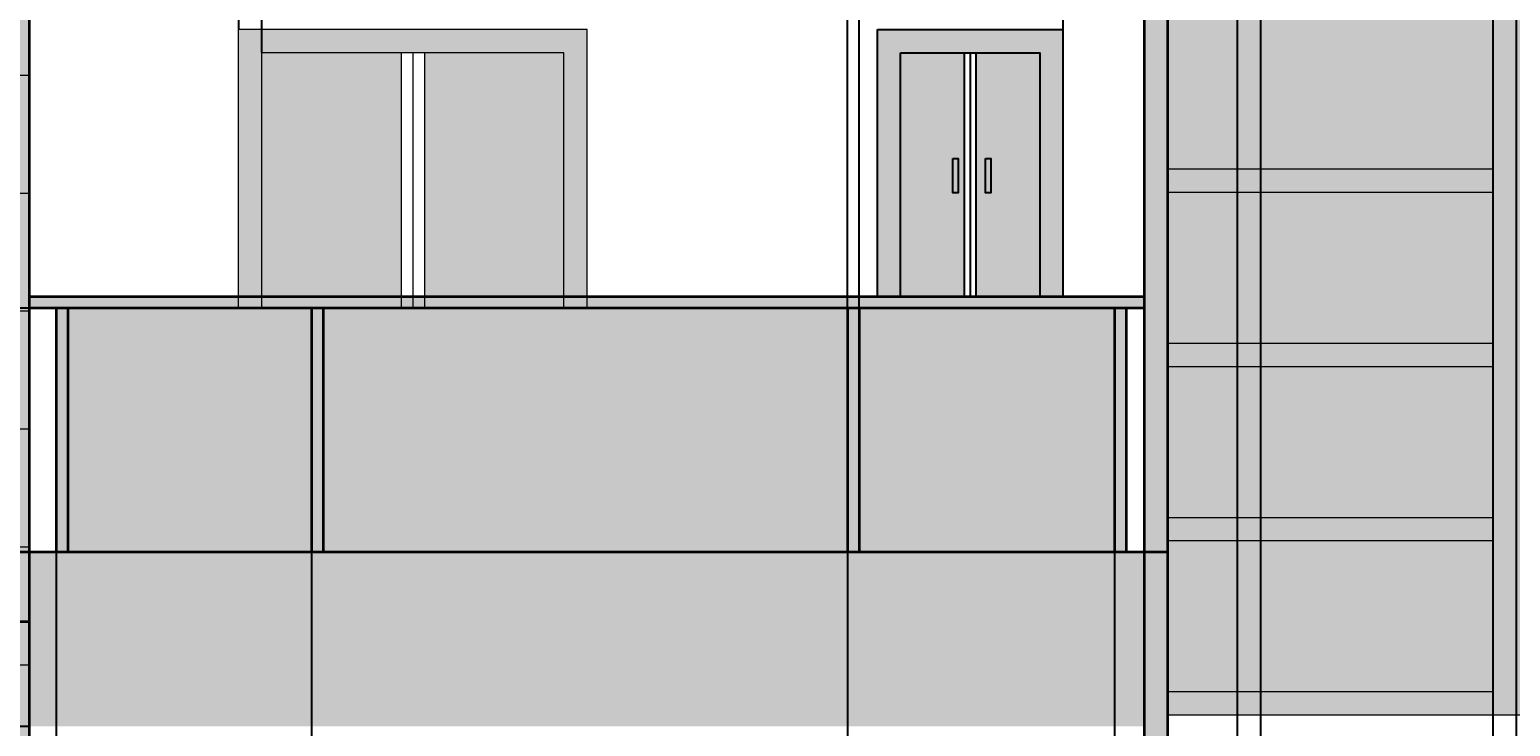
# Model space of a CAD drawing. Units: inches. Extents: x 2794 to 3619, y 522 to 1397.
# Tile 3 of 10: x 2954 to 3209, y 701 to 821. Entities that reach past the tile are written whole.
import ezdxf

# ---------------------------------------------------------------- set-up
doc = ezdxf.new("R2010")
doc.units = ezdxf.units.IN
for name, color, linetype, lineweight in [('A-ANNO-DIMS', 2, 'Continuous', 18), ('A-DOOR', 3, 'Continuous', 25), ('A-ELEV', 7, 'Continuous', 35), ('A-ELEV-PATT', 8, 'Continuous', 13), ('A-GLAZ', 4, 'Continuous', 18)]:
    doc.layers.add(name, color=color, linetype=linetype, lineweight=lineweight)
doc.styles.get("Standard").update_dxf_attribs({"font": 'arial.ttf'})
doc.dimstyles.get("Standard").update_dxf_attribs({"dimtxt": 0.18, "dimasz": 0.18, "dimexe": 0.18, "dimexo": 0.0625, "dimgap": 0.09, "dimtad": 0, "dimtih": 1, "dimtoh": 1, "dimdec": 4, "dimzin": 0, "dimdsep": 46, "dimtxsty": 'Standard', "dimcen": 0.09, "dimadec": 0, "dimazin": 0, "dimtfac": 1, "dimtdec": 4, "dimtofl": 0, "dimtmove": 0, "dimatfit": 3, "dimfxl": 1, "dimtolj": 1, "dimtzin": 0, "dimarcsym": 0})

# ---------------------------------------------------------------- blocks, each defined once
blk = doc.blocks.new('WIN-1500')
at = {"transparency": 33554646}
h = blk.add_hatch(color=256, dxfattribs=at)
h.dxf.hatch_style = 1
h.paths.add_polyline_path([(60, 48), (0, 48), (0, 2), (4, 2), (4, 44), (56, 44), (56, 2), (60, 2)])
at = {"transparency": 33554687}
h = blk.add_hatch(color=256, dxfattribs=at)
h.dxf.hatch_style = 1
h.set_gradient(color1=(248, 246, 176), color2=(74, 13, 14), name='INVCYLINDER')
h.paths.add_polyline_path([(56, 44), (32, 44), (32, 2), (56, 2)])
h.paths.add_polyline_path([(28, 44), (4, 44), (4, 2), (28, 2)])
for p, q in [((0, 0), (0, 48)), ((60, 48), (0, 48)), ((60, 0), (60, 48)), ((56, 44), (4, 44)), ((4, 0), (4, 44)), ((28, 44), (28, 0)), ((30, 44), (30, 0)), ((32, 44), (32, 0)), ((56, 0), (56, 44))]:
    blk.add_line(p, q)
blk = doc.blocks.new('DOOR-BALCONY-DBL')
at = {"transparency": 33554628}
h = blk.add_hatch(color=256, dxfattribs=at)
h.dxf.hatch_style = 1
h.paths.add_polyline_path([(4, 42), (28, 42), (28, 0), (32, 0), (32, 46), (0, 46), (0, 0), (4, 0)])
at = {"transparency": 33554646}
h = blk.add_hatch(color=256, dxfattribs=at)
h.dxf.hatch_style = 1
h.set_gradient(color1=(255, 255, 255), color2=(147, 149, 152), name='INVCYLINDER')
h.paths.add_polyline_path([(15, 42), (4, 42), (4, 0), (15, 0)])
h = blk.add_hatch(color=256, dxfattribs=at)
h.dxf.hatch_style = 1
h.set_gradient(color1=(255, 255, 255), color2=(147, 149, 152), name='INVCYLINDER')
h.paths.add_polyline_path([(28, 42), (17, 42), (17, 0), (28, 0)])
for p, q in [((0, 0), (0, 46)), ((0, 46), (32, 46)), ((4, 46), (28, 46)), ((32, 0), (32, 46)), ((4, 0), (4, 42)), ((4, 42), (28, 42)), ((15, 0), (15, 42)), ((16, 0), (16, 42)), ((17, 0), (17, 42)), ((28, 0), (28, 42))]:
    blk.add_line(p, q)
for points in [[(12.99, 23.83), (13.93, 23.83), (13.93, 17.87), (12.99, 17.87)], [(18.59, 23.83), (19.53, 23.83), (19.53, 17.87), (18.59, 17.87)]]:
    blk.add_lwpolyline(points, close=True)
blk = doc.blocks.new('*D16')
at = {"layer": 'A-ANNO-DIMS', "color": 0, "lineweight": -2, "transparency": 16777216}
for p, q in [((3142.2, 1356.64), (2793.99, 1356.64)), ((2794.17, 1356.46), (2794.17, 959.82)), ((2794.17, 562.82), (2794.17, 959.45)), ((2834.2, 562.64), (2793.99, 562.64))]:
    blk.add_line(p, q, dxfattribs=at)
at = {"layer": 'A-ANNO-DIMS', "color": 0, "transparency": 16777216}
for points in [[(2794.14, 1356.46), (2794.2, 1356.46), (2794.17, 1356.64)], [(2794.14, 562.82), (2794.2, 562.82), (2794.17, 562.64)]]:
    blk.add_solid(points, dxfattribs=at)
at = {"layer": 'Defpoints', "color": 0, "transparency": 16777216}
for p in [(2794.17, 1356.64), (3142.27, 1356.64), (2834.27, 562.64)]:
    blk.add_point(p, dxfattribs=at)
at = {"layer": 'A-ANNO-DIMS', "color": 0, "transparency": 16777216, "insert": (2794.17, 959.64), "char_height": 0.18, "attachment_point": 5}
blk.add_mtext('\\A1;794', dxfattribs=at)
blk = doc.blocks.new('*D29')
at = {"layer": 'A-ANNO-DIMS', "color": 0, "lineweight": -2, "transparency": 16777216}
for p, q in [((2990.27, 820.7), (2990.27, 1396.92)), ((2990.45, 1396.74), (2992.11, 1396.74)), ((2994.09, 1396.74), (2992.42, 1396.74)), ((2994.27, 816.7), (2994.27, 1396.92))]:
    blk.add_line(p, q, dxfattribs=at)
at = {"layer": 'A-ANNO-DIMS', "color": 0, "transparency": 16777216}
for points in [[(2990.45, 1396.77), (2990.45, 1396.71), (2990.27, 1396.74)], [(2994.09, 1396.77), (2994.09, 1396.71), (2994.27, 1396.74)]]:
    blk.add_solid(points, dxfattribs=at)
at = {"layer": 'Defpoints', "color": 0, "transparency": 16777216}
for p in [(2994.27, 1396.74), (2990.27, 820.64), (2994.27, 816.64)]:
    blk.add_point(p, dxfattribs=at)
at = {"layer": 'A-ANNO-DIMS', "color": 0, "transparency": 16777216, "insert": (2992.27, 1396.74), "char_height": 0.18, "attachment_point": 5}
blk.add_mtext('\\A1;4', dxfattribs=at)
blk = doc.blocks.new('*D31')
at = {"layer": 'A-ANNO-DIMS', "color": 0, "lineweight": -2, "transparency": 16777216}
for p, q in [((3132.27, 820.7), (3132.27, 1396.92)), ((3132.45, 1396.74), (3139.06, 1396.74)), ((3146.09, 1396.74), (3139.48, 1396.74)), ((3146.27, 774.7), (3146.27, 1396.92))]:
    blk.add_line(p, q, dxfattribs=at)
at = {"layer": 'A-ANNO-DIMS', "color": 0, "transparency": 16777216}
for points in [[(3132.45, 1396.77), (3132.45, 1396.71), (3132.27, 1396.74)], [(3146.09, 1396.77), (3146.09, 1396.71), (3146.27, 1396.74)]]:
    blk.add_solid(points, dxfattribs=at)
at = {"layer": 'Defpoints', "color": 0, "transparency": 16777216}
for p in [(3146.27, 1396.74), (3132.27, 820.64), (3146.27, 774.64)]:
    blk.add_point(p, dxfattribs=at)
at = {"layer": 'A-ANNO-DIMS', "color": 0, "transparency": 16777216, "insert": (3139.27, 1396.74), "char_height": 0.18, "attachment_point": 5}
blk.add_mtext('\\A1;14', dxfattribs=at)
blk = doc.blocks.new('*D32')
at = {"layer": 'A-ANNO-DIMS', "color": 0, "lineweight": -2, "transparency": 16777216}
for p, q in [((2954.27, 772.57), (2954.27, 522.36)), ((2958.83, 730.57), (2958.83, 522.36)), ((2954.45, 522.54), (2956.17, 522.54)), ((2958.65, 522.54), (2956.93, 522.54))]:
    blk.add_line(p, q, dxfattribs=at)
at = {"layer": 'A-ANNO-DIMS', "color": 0, "transparency": 16777216}
for points in [[(2954.45, 522.57), (2954.45, 522.51), (2954.27, 522.54)], [(2958.65, 522.57), (2958.65, 522.51), (2958.83, 522.54)]]:
    blk.add_solid(points, dxfattribs=at)
at = {"layer": 'Defpoints', "color": 0, "transparency": 16777216}
for p in [(2954.27, 772.64), (2958.83, 730.64), (2958.83, 522.54)]:
    blk.add_point(p, dxfattribs=at)
at = {"layer": 'A-ANNO-DIMS', "color": 0, "transparency": 16777216, "insert": (2956.55, 522.54), "char_height": 0.18, "attachment_point": 5}
blk.add_mtext('\\A1;4.561', dxfattribs=at)
blk = doc.blocks.new('*D33')
at = {"layer": 'A-ANNO-DIMS', "color": 0, "lineweight": -2, "transparency": 16777216}
for p, q in [((2958.83, 730.57), (2958.83, 522.36)), ((3002.83, 730.57), (3002.83, 522.36)), ((2959.01, 522.54), (2980.6, 522.54)), ((3002.65, 522.54), (2981.05, 522.54))]:
    blk.add_line(p, q, dxfattribs=at)
at = {"layer": 'A-ANNO-DIMS', "color": 0, "transparency": 16777216}
for points in [[(2959.01, 522.57), (2959.01, 522.51), (2958.83, 522.54)], [(3002.65, 522.57), (3002.65, 522.51), (3002.83, 522.54)]]:
    blk.add_solid(points, dxfattribs=at)
at = {"layer": 'Defpoints', "color": 0, "transparency": 16777216}
for p in [(2958.83, 730.64), (3002.83, 730.64), (3002.83, 522.54)]:
    blk.add_point(p, dxfattribs=at)
at = {"layer": 'A-ANNO-DIMS', "color": 0, "transparency": 16777216, "insert": (2980.83, 522.54), "char_height": 0.18, "attachment_point": 5}
blk.add_mtext('\\A1;44', dxfattribs=at)
blk = doc.blocks.new('*D34')
at = {"layer": 'A-ANNO-DIMS', "color": 0, "lineweight": -2, "transparency": 16777216}
for p, q in [((3002.83, 730.57), (3002.83, 522.36)), ((3095.13, 730.57), (3095.13, 522.36)), ((3003.01, 522.54), (3048.66, 522.54)), ((3094.95, 522.54), (3049.3, 522.54))]:
    blk.add_line(p, q, dxfattribs=at)
at = {"layer": 'A-ANNO-DIMS', "color": 0, "transparency": 16777216}
for points in [[(3003.01, 522.57), (3003.01, 522.51), (3002.83, 522.54)], [(3094.95, 522.57), (3094.95, 522.51), (3095.13, 522.54)]]:
    blk.add_solid(points, dxfattribs=at)
at = {"layer": 'Defpoints', "color": 0, "transparency": 16777216}
for p in [(3002.83, 730.64), (3095.13, 730.64), (3095.13, 522.54)]:
    blk.add_point(p, dxfattribs=at)
at = {"layer": 'A-ANNO-DIMS', "color": 0, "transparency": 16777216, "insert": (3048.98, 522.54), "char_height": 0.18, "attachment_point": 5}
blk.add_mtext('\\A1;92.3', dxfattribs=at)
blk = doc.blocks.new('*D35')
at = {"layer": 'A-ANNO-DIMS', "color": 0, "lineweight": -2, "transparency": 16777216}
for p, q in [((3095.13, 730.57), (3095.13, 522.36)), ((3141.11, 730.57), (3141.11, 522.36)), ((3095.31, 522.54), (3117.72, 522.54)), ((3140.93, 522.54), (3118.52, 522.54))]:
    blk.add_line(p, q, dxfattribs=at)
at = {"layer": 'A-ANNO-DIMS', "color": 0, "transparency": 16777216}
for points in [[(3095.31, 522.57), (3095.31, 522.51), (3095.13, 522.54)], [(3140.93, 522.57), (3140.93, 522.51), (3141.11, 522.54)]]:
    blk.add_solid(points, dxfattribs=at)
at = {"layer": 'Defpoints', "color": 0, "transparency": 16777216}
for p in [(3095.13, 730.64), (3141.11, 730.64), (3141.11, 522.54)]:
    blk.add_point(p, dxfattribs=at)
at = {"layer": 'A-ANNO-DIMS', "color": 0, "transparency": 16777216, "insert": (3118.12, 522.54), "char_height": 0.18, "attachment_point": 5}
blk.add_mtext('\\A1;45.98', dxfattribs=at)
blk = doc.blocks.new('*D36')
at = {"layer": 'A-ANNO-DIMS', "color": 0, "lineweight": -2, "transparency": 16777216}
for p, q in [((3146.27, 772.57), (3146.27, 522.36)), ((3141.11, 730.57), (3141.11, 522.36)), ((3141.29, 522.54), (3143.3, 522.54)), ((3146.09, 522.54), (3144.08, 522.54))]:
    blk.add_line(p, q, dxfattribs=at)
at = {"layer": 'A-ANNO-DIMS', "color": 0, "transparency": 16777216}
for points in [[(3141.29, 522.57), (3141.29, 522.51), (3141.11, 522.54)], [(3146.09, 522.57), (3146.09, 522.51), (3146.27, 522.54)]]:
    blk.add_solid(points, dxfattribs=at)
at = {"layer": 'Defpoints', "color": 0, "transparency": 16777216}
for p in [(3146.27, 772.64), (3141.11, 730.64), (3146.27, 522.54)]:
    blk.add_point(p, dxfattribs=at)
at = {"layer": 'A-ANNO-DIMS', "color": 0, "transparency": 16777216, "insert": (3143.69, 522.54), "char_height": 0.18, "attachment_point": 5}
blk.add_mtext('\\A1;5.154', dxfattribs=at)
blk = doc.blocks.new('*D37')
at = {"layer": 'A-ANNO-DIMS', "color": 0, "lineweight": -2, "transparency": 16777216}
for p, q in [((3095.13, 772.7), (3095.13, 1396.92)), ((3095.31, 1396.74), (3095.98, 1396.74)), ((3096.95, 1396.74), (3096.28, 1396.74)), ((3097.13, 772.7), (3097.13, 1396.92))]:
    blk.add_line(p, q, dxfattribs=at)
at = {"layer": 'A-ANNO-DIMS', "color": 0, "transparency": 16777216}
for points in [[(3095.31, 1396.77), (3095.31, 1396.71), (3095.13, 1396.74)], [(3096.95, 1396.77), (3096.95, 1396.71), (3097.13, 1396.74)]]:
    blk.add_solid(points, dxfattribs=at)
at = {"layer": 'Defpoints', "color": 0, "transparency": 16777216}
for p in [(3097.13, 1396.74), (3095.13, 772.64), (3097.13, 772.64)]:
    blk.add_point(p, dxfattribs=at)
at = {"layer": 'A-ANNO-DIMS', "color": 0, "transparency": 16777216, "insert": (3096.13, 1396.74), "char_height": 0.18, "attachment_point": 5}
blk.add_mtext('\\A1;2', dxfattribs=at)
blk = doc.blocks.new('*D38')
at = {"layer": 'A-ANNO-DIMS', "color": 0, "lineweight": -2, "transparency": 16777216}
for p, q in [((2958.76, 730.64), (2793.99, 730.64)), ((2794.17, 730.46), (2794.17, 715.82)), ((2794.17, 700.82), (2794.17, 715.45)), ((2954.2, 700.64), (2793.99, 700.64))]:
    blk.add_line(p, q, dxfattribs=at)
at = {"layer": 'A-ANNO-DIMS', "color": 0, "transparency": 16777216}
for points in [[(2794.14, 730.46), (2794.2, 730.46), (2794.17, 730.64)], [(2794.14, 700.82), (2794.2, 700.82), (2794.17, 700.64)]]:
    blk.add_solid(points, dxfattribs=at)
at = {"layer": 'Defpoints', "color": 0, "transparency": 16777216}
for p in [(2794.17, 730.64), (2958.83, 730.64), (2954.27, 700.64)]:
    blk.add_point(p, dxfattribs=at)
at = {"layer": 'A-ANNO-DIMS', "color": 0, "transparency": 16777216, "insert": (2794.17, 715.64), "char_height": 0.18, "attachment_point": 5}
blk.add_mtext('\\A1;30', dxfattribs=at)
blk = doc.blocks.new('*D39')
at = {"layer": 'A-ANNO-DIMS', "color": 0, "lineweight": -2, "transparency": 16777216}
for p, q in [((2954.2, 772.64), (2793.99, 772.64)), ((2794.17, 772.46), (2794.17, 751.82)), ((2794.17, 730.82), (2794.17, 751.45)), ((2958.76, 730.64), (2793.99, 730.64))]:
    blk.add_line(p, q, dxfattribs=at)
at = {"layer": 'A-ANNO-DIMS', "color": 0, "transparency": 16777216}
for points in [[(2794.14, 772.46), (2794.2, 772.46), (2794.17, 772.64)], [(2794.14, 730.82), (2794.2, 730.82), (2794.17, 730.64)]]:
    blk.add_solid(points, dxfattribs=at)
at = {"layer": 'Defpoints', "color": 0, "transparency": 16777216}
for p in [(2794.17, 772.64), (2954.27, 772.64), (2958.83, 730.64)]:
    blk.add_point(p, dxfattribs=at)
at = {"layer": 'A-ANNO-DIMS', "color": 0, "transparency": 16777216, "insert": (2794.17, 751.64), "char_height": 0.18, "attachment_point": 5}
blk.add_mtext('\\A1;42', dxfattribs=at)
blk = doc.blocks.new('*D49')
at = {"layer": 'A-ANNO-DIMS', "color": 0, "lineweight": -2, "transparency": 16777216}
for p, q in [((3146.27, 1256.19), (3146.27, 522.36)), ((3150.27, 1254.57), (3150.27, 522.36)), ((3146.45, 522.54), (3148.11, 522.54)), ((3150.09, 522.54), (3148.42, 522.54))]:
    blk.add_line(p, q, dxfattribs=at)
at = {"layer": 'A-ANNO-DIMS', "color": 0, "transparency": 16777216}
for points in [[(3146.45, 522.57), (3146.45, 522.51), (3146.27, 522.54)], [(3150.09, 522.57), (3150.09, 522.51), (3150.27, 522.54)]]:
    blk.add_solid(points, dxfattribs=at)
at = {"layer": 'Defpoints', "color": 0, "transparency": 16777216}
for p in [(3146.27, 1256.25), (3150.27, 1254.64), (3150.27, 522.54)]:
    blk.add_point(p, dxfattribs=at)
at = {"layer": 'A-ANNO-DIMS', "color": 0, "transparency": 16777216, "insert": (3148.27, 522.54), "char_height": 0.18, "attachment_point": 5}
blk.add_mtext('\\A1;4', dxfattribs=at)
blk = doc.blocks.new('*D50')
at = {"layer": 'A-ANNO-DIMS', "color": 0, "lineweight": -2, "transparency": 16777216}
for p, q in [((3150.27, 1254.57), (3150.27, 522.36)), ((3206.27, 1254.57), (3206.27, 522.36)), ((3150.45, 522.54), (3178.05, 522.54)), ((3206.09, 522.54), (3178.48, 522.54))]:
    blk.add_line(p, q, dxfattribs=at)
at = {"layer": 'A-ANNO-DIMS', "color": 0, "transparency": 16777216}
for points in [[(3150.45, 522.57), (3150.45, 522.51), (3150.27, 522.54)], [(3206.09, 522.57), (3206.09, 522.51), (3206.27, 522.54)]]:
    blk.add_solid(points, dxfattribs=at)
at = {"layer": 'Defpoints', "color": 0, "transparency": 16777216}
for p in [(3150.27, 1254.64), (3206.27, 1254.64), (3206.27, 522.54)]:
    blk.add_point(p, dxfattribs=at)
at = {"layer": 'A-ANNO-DIMS', "color": 0, "transparency": 16777216, "insert": (3178.27, 522.54), "char_height": 0.18, "attachment_point": 5}
blk.add_mtext('\\A1;56', dxfattribs=at)
blk = doc.blocks.new('*D51')
at = {"layer": 'A-ANNO-DIMS', "color": 0, "lineweight": -2, "transparency": 16777216}
for p, q in [((3206.27, 1254.57), (3206.27, 522.36)), ((3210.27, 1254.57), (3210.27, 522.36)), ((3206.45, 522.54), (3208.11, 522.54)), ((3210.09, 522.54), (3208.42, 522.54))]:
    blk.add_line(p, q, dxfattribs=at)
at = {"layer": 'A-ANNO-DIMS', "color": 0, "transparency": 16777216}
for points in [[(3206.45, 522.57), (3206.45, 522.51), (3206.27, 522.54)], [(3210.09, 522.57), (3210.09, 522.51), (3210.27, 522.54)]]:
    blk.add_solid(points, dxfattribs=at)
at = {"layer": 'Defpoints', "color": 0, "transparency": 16777216}
for p in [(3206.27, 1254.64), (3210.27, 1254.64), (3210.27, 522.54)]:
    blk.add_point(p, dxfattribs=at)
at = {"layer": 'A-ANNO-DIMS', "color": 0, "transparency": 16777216, "insert": (3208.27, 522.54), "char_height": 0.18, "attachment_point": 5}
blk.add_mtext('\\A1;4', dxfattribs=at)
blk = doc.blocks.new('*D56')
at = {"layer": 'A-ANNO-DIMS', "color": 0, "lineweight": -2, "transparency": 16777216}
for p, q in [((3162.27, 664.7), (3162.27, 1396.92)), ((3162.45, 1396.74), (3206.05, 1396.74)), ((3250.09, 1396.74), (3206.49, 1396.74)), ((3250.27, 664.7), (3250.27, 1396.92))]:
    blk.add_line(p, q, dxfattribs=at)
at = {"layer": 'A-ANNO-DIMS', "color": 0, "transparency": 16777216}
for points in [[(3162.45, 1396.77), (3162.45, 1396.71), (3162.27, 1396.74)], [(3250.09, 1396.77), (3250.09, 1396.71), (3250.27, 1396.74)]]:
    blk.add_solid(points, dxfattribs=at)
at = {"layer": 'Defpoints', "color": 0, "transparency": 16777216}
for p in [(3250.27, 1396.74), (3162.27, 664.64), (3250.27, 664.64)]:
    blk.add_point(p, dxfattribs=at)
at = {"layer": 'A-ANNO-DIMS', "color": 0, "transparency": 16777216, "insert": (3206.27, 1396.74), "char_height": 0.18, "attachment_point": 5}
blk.add_mtext('\\A1;88', dxfattribs=at)
blk = doc.blocks.new('*D57')
at = {"layer": 'A-ANNO-DIMS', "color": 0, "lineweight": -2, "transparency": 16777216}
for p, q in [((3162.27, 664.7), (3162.27, 1396.92)), ((3162.45, 1396.74), (3164.11, 1396.74)), ((3166.09, 1396.74), (3164.42, 1396.74)), ((3166.27, 660.7), (3166.27, 1396.92))]:
    blk.add_line(p, q, dxfattribs=at)
at = {"layer": 'A-ANNO-DIMS', "color": 0, "transparency": 16777216}
for points in [[(3162.45, 1396.77), (3162.45, 1396.71), (3162.27, 1396.74)], [(3166.09, 1396.77), (3166.09, 1396.71), (3166.27, 1396.74)]]:
    blk.add_solid(points, dxfattribs=at)
at = {"layer": 'Defpoints', "color": 0, "transparency": 16777216}
for p in [(3166.27, 1396.74), (3162.27, 664.64), (3166.27, 660.64)]:
    blk.add_point(p, dxfattribs=at)
at = {"layer": 'A-ANNO-DIMS', "color": 0, "transparency": 16777216, "insert": (3164.27, 1396.74), "char_height": 0.18, "attachment_point": 5}
blk.add_mtext('\\A1;4', dxfattribs=at)
blk = doc.blocks.new('*D58')
at = {"layer": 'A-ANNO-DIMS', "color": 0, "lineweight": -2, "transparency": 16777216}
for p, q in [((3150.27, 580.7), (3150.27, 1396.92)), ((3150.45, 1396.74), (3156.06, 1396.74)), ((3162.09, 1396.74), (3156.48, 1396.74)), ((3162.27, 664.7), (3162.27, 1396.92))]:
    blk.add_line(p, q, dxfattribs=at)
at = {"layer": 'A-ANNO-DIMS', "color": 0, "transparency": 16777216}
for points in [[(3150.45, 1396.77), (3150.45, 1396.71), (3150.27, 1396.74)], [(3162.09, 1396.77), (3162.09, 1396.71), (3162.27, 1396.74)]]:
    blk.add_solid(points, dxfattribs=at)
at = {"layer": 'Defpoints', "color": 0, "transparency": 16777216}
for p in [(3162.27, 1396.74), (3162.27, 664.64), (3150.27, 580.64)]:
    blk.add_point(p, dxfattribs=at)
at = {"layer": 'A-ANNO-DIMS', "color": 0, "transparency": 16777216, "insert": (3156.27, 1396.74), "char_height": 0.18, "attachment_point": 5}
blk.add_mtext('\\A1;12', dxfattribs=at)

msp = doc.modelspace()

# ---------------------------------------------------------------- hatches: boundary and pattern name
at = {"layer": 'A-ELEV-PATT', "transparency": 33554687}
h = msp.add_hatch(color=256, dxfattribs=at)
h.dxf.hatch_style = 1
h.paths.add_polyline_path([(3262.2659, 1350.6351), (3150.2659, 1350.6351), (3150.2659, 1279.0155, -0.68639605), (3262.2659, 1279.0155)])
h.paths.add_polyline_path([(3210.2659, 1314.1121), (3210.2659, 1258.6351), (3262.2659, 1258.6351, 0.39146256)])
h.paths.add_polyline_path([(3206.2659, 1314.2551, 0.41222069), (3150.2659, 1258.6351), (3206.2659, 1258.6351)])
h.paths.add_polyline_path([(3262.2659, 1254.6351), (3210.2659, 1254.6351), (3210.2659, 1216.6351), (3262.2659, 1216.6351)])
h.paths.add_polyline_path([(3206.2659, 1254.6351), (3150.2659, 1254.6351), (3150.2659, 1216.6351), (3206.2659, 1216.6351)])
h.paths.add_polyline_path([(3262.2659, 1212.6351), (3210.2659, 1212.6351), (3210.2659, 1186.6351), (3262.2659, 1186.6351)])
h.paths.add_polyline_path([(3206.2659, 1212.6351), (3150.2659, 1212.6351), (3150.2659, 1186.6351), (3206.2659, 1186.6351)])
h.paths.add_polyline_path([(3206.2659, 1182.6351), (3150.2659, 1182.6351), (3150.2659, 1156.6351), (3206.2659, 1156.6351)])
h.paths.add_polyline_path([(3262.2659, 1182.6351), (3210.2659, 1182.6351), (3210.2659, 1156.6351), (3262.2659, 1156.6351)])
h.paths.add_polyline_path([(3262.2659, 1152.6351), (3210.2659, 1152.6351), (3210.2659, 1126.6351), (3262.2659, 1126.6351)])
h.paths.add_polyline_path([(3206.2659, 1152.6351), (3150.2659, 1152.6351), (3150.2659, 1126.6351), (3206.2659, 1126.6351)])
h.paths.add_polyline_path([(3262.2659, 1122.6351), (3210.2659, 1122.6351), (3210.2659, 1096.6351), (3262.2659, 1096.6351)])
h.paths.add_polyline_path([(3206.2659, 1122.6351), (3150.2659, 1122.6351), (3150.2659, 1096.6351), (3206.2659, 1096.6351)])
h.paths.add_polyline_path([(3206.2659, 1092.6351), (3150.2659, 1092.6351), (3150.2659, 1066.6351), (3206.2659, 1066.6351)])
h.paths.add_polyline_path([(3262.2659, 1092.6351), (3210.2659, 1092.6351), (3210.2659, 1066.6351), (3262.2659, 1066.6351)])
h.paths.add_polyline_path([(3262.2659, 1062.6351), (3210.2659, 1062.6351), (3210.2659, 1036.6351), (3262.2659, 1036.6351)])
h.paths.add_polyline_path([(3206.2659, 1062.6351), (3150.2659, 1062.6351), (3150.2659, 1036.6351), (3206.2659, 1036.6351)])
h.paths.add_polyline_path([(3206.2659, 1032.6351), (3150.2659, 1032.6351), (3150.2659, 1006.6351), (3206.2659, 1006.6351)])
h.paths.add_polyline_path([(3262.2659, 1032.6351), (3210.2659, 1032.6351), (3210.2659, 1006.6351), (3262.2659, 1006.6351)])
h.paths.add_polyline_path([(3262.2659, 1002.6351), (3210.2659, 1002.6351), (3210.2659, 976.6351), (3262.2659, 976.6351)])
h.paths.add_polyline_path([(3206.2659, 1002.6351), (3150.2659, 1002.6351), (3150.2659, 976.6351), (3206.2659, 976.6351)])
h.paths.add_polyline_path([(3206.2659, 972.6351), (3150.2659, 972.6351), (3150.2659, 946.6351), (3206.2659, 946.6351)])
h.paths.add_polyline_path([(3206.2659, 942.6351), (3150.2659, 942.6351), (3150.2659, 916.6351), (3206.2659, 916.6351)])
h.paths.add_polyline_path([(3262.2659, 942.6351), (3210.2659, 942.6351), (3210.2659, 916.6351), (3262.2659, 916.6351)])
h.paths.add_polyline_path([(3262.2659, 972.6351), (3210.2659, 972.6351), (3210.2659, 946.6351), (3262.2659, 946.6351)])
h.paths.add_polyline_path([(3262.2659, 912.6351), (3210.2659, 912.6351), (3210.2659, 886.6351), (3262.2659, 886.6351)])
h.paths.add_polyline_path([(3206.2659, 912.6351), (3150.2659, 912.6351), (3150.2659, 886.6351), (3206.2659, 886.6351)])
h.paths.add_polyline_path([(3206.2659, 882.6351), (3150.2659, 882.6351), (3150.2659, 856.6351), (3206.2659, 856.6351)])
h.paths.add_polyline_path([(3262.2659, 882.6351), (3210.2659, 882.6351), (3210.2659, 856.6351), (3262.2659, 856.6351)])
h.paths.add_polyline_path([(3262.2659, 852.6351), (3210.2659, 852.6351), (3210.2659, 826.6351), (3262.2659, 826.6351)])
h.paths.add_polyline_path([(3206.2659, 852.6351), (3150.2659, 852.6351), (3150.2659, 826.6351), (3206.2659, 826.6351)])
h.paths.add_polyline_path([(3206.2659, 822.6351), (3150.2659, 822.6351), (3150.2659, 796.6351), (3206.2659, 796.6351)])
h.paths.add_polyline_path([(3262.2659, 822.6351), (3210.2659, 822.6351), (3210.2659, 796.6351), (3262.2659, 796.6351)])
h.paths.add_polyline_path([(3262.2659, 792.6351), (3210.2659, 792.6351), (3210.2659, 766.6351), (3262.2659, 766.6351)])
h.paths.add_polyline_path([(3206.2659, 792.6351), (3150.2659, 792.6351), (3150.2659, 766.6351), (3206.2659, 766.6351)])
h.paths.add_polyline_path([(3206.2659, 762.6351), (3150.2659, 762.6351), (3150.2659, 736.6351), (3206.2659, 736.6351)])
h.paths.add_polyline_path([(3206.2659, 732.6351), (3150.2659, 732.6351), (3150.2659, 706.6351), (3206.2659, 706.6351)])
h.paths.add_polyline_path([(3262.2659, 732.6351), (3210.2659, 732.6351), (3210.2659, 706.6351), (3262.2659, 706.6351)])
h.paths.add_polyline_path([(3262.2659, 762.6351), (3210.2659, 762.6351), (3210.2659, 736.6351), (3262.2659, 736.6351)])
h = msp.add_hatch(color=256, dxfattribs=at)
h.dxf.hatch_style = 1
h.paths.add_polyline_path([(3150.2659, 1257.8725, -0.00340445), (3150.2659, 1258.6351), (3146.2659, 1258.6351), (3146.2659, 1228.6351), (3150.2659, 1228.6351)])
h.paths.add_polyline_path([(3262.2659, 1258.6351), (3210.2659, 1258.6351), (3210.2659, 1314.1121, 0.01787385), (3206.2659, 1314.2551), (3206.2659, 1258.6351), (3150.2659, 1258.6351), (3150.2659, 1254.6351), (3206.2659, 1254.6351), (3206.2659, 1216.6351), (3150.2659, 1216.6351), (3150.2659, 1212.6351), (3206.2659, 1212.6351), (3206.2659, 1186.6351), (3150.2659, 1186.6351), (3150.2659, 1182.6351), (3206.2659, 1182.6351), (3206.2659, 1156.6351), (3150.2659, 1156.6351), (3150.2659, 1152.6351), (3206.2659, 1152.6351), (3206.2659, 1126.6351), (3150.2659, 1126.6351), (3150.2659, 1122.6351), (3206.2659, 1122.6351), (3206.2659, 1096.6351), (3150.2659, 1096.6351), (3150.2659, 1092.6351), (3206.2659, 1092.6351), (3206.2659, 1066.6351), (3150.2659, 1066.6351), (3150.2659, 1062.6351), (3206.2659, 1062.6351), (3206.2659, 1036.6351), (3150.2659, 1036.6351), (3150.2659, 1032.6351), (3206.2659, 1032.6351), (3206.2659, 1006.6351), (3150.2659, 1006.6351), (3150.2659, 1002.6351), (3206.2659, 1002.6351), (3206.2659, 976.6351), (3150.2659, 976.6351), (3150.2659, 972.6351), (3206.2659, 972.6351), (3206.2659, 946.6351), (3150.2659, 946.6351), (3150.2659, 942.6351), (3206.2659, 942.6351), (3206.2659, 916.6351), (3150.2659, 916.6351), (3150.2659, 912.6351), (3206.2659, 912.6351), (3206.2659, 886.6351), (3150.2659, 886.6351), (3150.2659, 882.6351), (3206.2659, 882.6351), (3206.2659, 856.6351), (3150.2659, 856.6351), (3150.2659, 852.6351), (3206.2659, 852.6351), (3206.2659, 826.6351), (3150.2659, 826.6351), (3150.2659, 822.6351), (3206.2659, 822.6351), (3206.2659, 796.6351), (3150.2659, 796.6351), (3150.2659, 792.6351), (3206.2659, 792.6351), (3206.2659, 766.6351), (3150.2659, 766.6351), (3150.2659, 762.6351), (3206.2659, 762.6351), (3206.2659, 736.6351), (3150.2659, 736.6351), (3150.2659, 732.6351), (3206.2659, 732.6351), (3206.2659, 706.6351), (3150.2659, 706.6351), (3150.2659, 702.6351), (3262.2659, 702.6351), (3262.2659, 706.6351), (3210.2659, 706.6351), (3210.2659, 732.6351), (3262.2659, 732.6351), (3262.2659, 736.6351), (3210.2659, 736.6351), (3210.2659, 762.6351), (3262.2659, 762.6351), (3262.2659, 766.6351), (3210.2659, 766.6351), (3210.2659, 792.6351), (3262.2659, 792.6351), (3262.2659, 796.6351), (3210.2659, 796.6351), (3210.2659, 822.6351), (3262.2659, 822.6351), (3262.2659, 826.6351), (3210.2659, 826.6351), (3210.2659, 852.6351), (3262.2659, 852.6351), (3262.2659, 856.6351), (3210.2659, 856.6351), (3210.2659, 882.6351), (3262.2659, 882.6351), (3262.2659, 886.6351), (3210.2659, 886.6351), (3210.2659, 912.6351), (3262.2659, 912.6351), (3262.2659, 916.6351), (3210.2659, 916.6351), (3210.2659, 942.6351), (3262.2659, 942.6351), (3262.2659, 946.6351), (3210.2659, 946.6351), (3210.2659, 972.6351), (3262.2659, 972.6351), (3262.2659, 976.6351), (3210.2659, 976.6351), (3210.2659, 1002.6351), (3262.2659, 1002.6351), (3262.2659, 1006.6351), (3210.2659, 1006.6351), (3210.2659, 1032.6351), (3262.2659, 1032.6351), (3262.2659, 1036.6351), (3210.2659, 1036.6351), (3210.2659, 1062.6351), (3262.2659, 1062.6351), (3262.2659, 1066.6351), (3210.2659, 1066.6351), (3210.2659, 1092.6351), (3262.2659, 1092.6351), (3262.2659, 1096.6351), (3210.2659, 1096.6351), (3210.2659, 1122.6351), (3262.2659, 1122.6351), (3262.2659, 1126.6351), (3210.2659, 1126.6351), (3210.2659, 1152.6351), (3262.2659, 1152.6351), (3262.2659, 1156.6351), (3210.2659, 1156.6351), (3210.2659, 1182.6351), (3262.2659, 1182.6351), (3262.2659, 1186.6351), (3210.2659, 1186.6351), (3210.2659, 1212.6351), (3262.2659, 1212.6351), (3262.2659, 1216.6351), (3210.2659, 1216.6351), (3210.2659, 1254.6351), (3262.2659, 1254.6351)])
h = msp.add_hatch(color=256, dxfattribs=at)
h.dxf.hatch_style = 1
h.paths.add_polyline_path([(2852.2659, 1246.6351), (2954.2659, 1246.6351), (2954.2659, 1258.6351), (2900.2659, 1258.6351), (2900.2659, 1294.6351), (2852.2659, 1294.6351)])
h.paths.add_polyline_path([(3512.2659, 1294.6351), (3512.2659, 1258.6351), (3458.2659, 1258.6351), (3458.2659, 1246.6351), (3560.2659, 1246.6351), (3560.2659, 1294.6351)])
h.paths.add_polyline_path([(2954.2659, 1114.6351), (2954.2659, 1126.6351), (2852.2659, 1126.6351), (2852.2659, 1114.6351)])
h.paths.add_polyline_path([(3560.2659, 1114.6351), (3560.2659, 1126.6351), (3458.2659, 1126.6351), (3458.2659, 1114.6351)])
h.paths.add_polyline_path([(3560.2659, 982.6351), (3560.2659, 994.6351), (3458.2659, 994.6351), (3458.2659, 982.6351)])
h.paths.add_polyline_path([(2954.2659, 982.6351), (2954.2659, 994.6351), (2852.2659, 994.6351), (2852.2659, 982.6351)])
h.paths.add_polyline_path([(2852.2659, 862.6351), (2852.2659, 850.6351), (2954.2659, 850.6351), (2954.2659, 862.6351)])
h.paths.add_polyline_path([(2852.2659, 730.6351), (2852.2659, 718.6351), (2954.2659, 718.6351), (2954.2659, 730.6351)])
h.paths.add_polyline_path([(3560.2659, 718.6351), (3560.2659, 730.6351), (3458.2659, 730.6351), (3458.2659, 718.6351)])
h.paths.add_polyline_path([(3560.2659, 850.6351), (3560.2659, 862.6351), (3458.2659, 862.6351), (3458.2659, 850.6351)])
h = msp.add_hatch(color=256, dxfattribs=at)
h.dxf.hatch_style = 1
h.paths.add_polyline_path([(3146.2659, 1096.6351), (3146.2659, 1126.6351), (2954.2659, 1126.6351), (2954.2659, 1096.6351)])
h.paths.add_polyline_path([(3458.2659, 1096.6351), (3458.2659, 1126.6351), (3266.2659, 1126.6351), (3266.2659, 1096.6351)])
h.paths.add_polyline_path([(3458.2659, 964.6351), (3458.2659, 994.6351), (3266.2659, 994.6351), (3266.2659, 964.6351)])
h.paths.add_polyline_path([(3146.2659, 964.6351), (3146.2659, 994.6351), (2954.2659, 994.6351), (2954.2659, 964.6351)])
h.paths.add_polyline_path([(3458.2659, 832.6351), (3458.2659, 862.6351), (3266.2659, 862.6351), (3266.2659, 832.6351)])
h.paths.add_polyline_path([(3146.2659, 832.6351), (3146.2659, 862.6351), (2954.2659, 862.6351), (2954.2659, 832.6351)])
h.paths.add_polyline_path([(3458.2659, 700.6351), (3458.2659, 730.6351), (3266.2659, 730.6351), (3266.2659, 700.6351)])
h.paths.add_polyline_path([(3146.2659, 700.6351), (3146.2659, 730.6351), (2954.2659, 730.6351), (2954.2659, 700.6351)])
h.paths.add_polyline_path([(3266.2659, 1294.6351), (3266.2659, 1258.6351), (3266.2659, 1228.6351), (3458.2659, 1228.6351), (3458.2659, 1294.6351)])
h.paths.add_polyline_path([(3146.2659, 1228.6351), (3146.2659, 1256.2485, -0.00994307), (3146.2659, 1258.6351), (3146.2659, 1294.6351), (2954.2659, 1294.6351), (2954.2659, 1228.6351)])
at = {"layer": 'A-ELEV-PATT'}
h = msp.add_hatch(dxfattribs=at)
h.set_pattern_fill('AR-B816', color=256, scale=0.1)
h.paths.add_polyline_path([(2954.2659, 1114.6351), (2852.2659, 1114.6351), (2852.2659, 994.6351), (2954.2659, 994.6351)])
h.paths.add_polyline_path([(2954.2659, 1246.6351), (2852.2659, 1246.6351), (2852.2659, 1126.6351), (2954.2659, 1126.6351)])
h.paths.add_polyline_path([(2954.2659, 982.6351), (2852.2659, 982.6351), (2852.2659, 862.6351), (2954.2659, 862.6351)])
h.paths.add_polyline_path([(2954.2659, 850.6351), (2852.2659, 850.6351), (2852.2659, 730.6351), (2954.2659, 730.6351)])
h.paths.add_polyline_path([(3560.2659, 850.6351), (3458.2659, 850.6351), (3458.2659, 730.6351), (3560.2659, 730.6351)])
h.paths.add_polyline_path([(3560.2659, 982.6351), (3458.2659, 982.6351), (3458.2659, 862.6351), (3560.2659, 862.6351)])
h.paths.add_polyline_path([(3560.2659, 1114.6351), (3458.2659, 1114.6351), (3458.2659, 994.6351), (3560.2659, 994.6351)])
h.paths.add_polyline_path([(3560.2659, 1246.6351), (3458.2659, 1246.6351), (3458.2659, 1126.6351), (3560.2659, 1126.6351)])
h.paths.add_polyline_path([(2852.2659, 642.6351), (2954.2659, 642.6351), (2954.2659, 718.6351), (2852.2659, 718.6351)])
h.paths.add_polyline_path([(3458.2659, 640.6351), (3560.2659, 640.6351), (3560.2659, 718.6351), (3458.2659, 718.6351)])
at = {"layer": 'A-ELEV-PATT', "transparency": 33554630}
h = msp.add_hatch(color=256, dxfattribs=at)
h.dxf.hatch_style = 1
h.paths.add_polyline_path([(2954.2659, 1114.6351), (2852.2659, 1114.6351), (2852.2659, 994.6351), (2954.2659, 994.6351)])
h.paths.add_polyline_path([(2954.2659, 982.6351), (2852.2659, 982.6351), (2852.2659, 862.6351), (2954.2659, 862.6351)])
h.paths.add_polyline_path([(2954.2659, 850.6351), (2852.2659, 850.6351), (2852.2659, 730.6351), (2954.2659, 730.6351)])
h.paths.add_polyline_path([(3560.2659, 850.6351), (3458.2659, 850.6351), (3458.2659, 730.6351), (3560.2659, 730.6351)])
h.paths.add_polyline_path([(3560.2659, 982.6351), (3458.2659, 982.6351), (3458.2659, 862.6351), (3560.2659, 862.6351)])
h.paths.add_polyline_path([(3560.2659, 1114.6351), (3458.2659, 1114.6351), (3458.2659, 994.6351), (3560.2659, 994.6351)])
h.paths.add_polyline_path([(3560.2659, 1246.6351), (3458.2659, 1246.6351), (3458.2659, 1126.6351), (3560.2659, 1126.6351)])
h.paths.add_polyline_path([(2852.2659, 642.6351), (2954.2659, 642.6351), (2954.2659, 718.6351), (2852.2659, 718.6351)])
h.paths.add_polyline_path([(3458.2659, 642.6351), (3560.2659, 642.6351), (3560.2659, 718.6351), (3458.2659, 718.6351)])
at = {"layer": 'A-ELEV-PATT', "transparency": 33554687}
h = msp.add_hatch(color=256, dxfattribs=at)
h.dxf.hatch_style = 1
h.paths.add_polyline_path([(3150.2659, 1228.6351), (3146.2659, 1228.6351), (3146.2659, 1126.6351), (3150.2659, 1126.6351)])
h.paths.add_polyline_path([(3150.2659, 1126.6351), (3146.2659, 1126.6351), (3146.2659, 1038.6351), (3150.2659, 1038.6351)])
h.paths.add_polyline_path([(3150.2659, 1038.6351), (3146.2659, 1038.6351), (3146.2659, 964.6351), (3150.2659, 964.6351)])
h.paths.add_polyline_path([(3150.2659, 964.6351), (3146.2659, 964.6351), (3146.2659, 906.6351), (3150.2659, 906.6351)])
h.paths.add_polyline_path([(3150.2659, 906.6351), (3146.2659, 906.6351), (3146.2659, 832.6351), (3150.2659, 832.6351)])
h.paths.add_polyline_path([(3150.2659, 832.6351), (3146.2659, 832.6351), (3146.2659, 730.6351), (3150.2659, 730.6351)])
h = msp.add_hatch(color=256, dxfattribs=at)
h.dxf.hatch_style = 1
h.paths.add_polyline_path([(3146.2659, 772.6351), (3146.2659, 774.6351), (2954.2659, 774.6351), (2954.2659, 772.6351)])
h.paths.add_polyline_path([(3002.8268, 730.6351), (3004.8268, 730.6351), (3004.8268, 772.6351), (3002.8268, 772.6351)])
h.paths.add_polyline_path([(2958.8268, 730.6351), (2960.8268, 730.6351), (2960.8268, 772.6351), (2958.8268, 772.6351)])
h.paths.add_polyline_path([(3097.1329, 772.6351), (3095.1329, 772.6351), (3095.1329, 730.6351), (3097.1329, 730.6351)])
h.paths.add_polyline_path([(3141.112, 730.6351), (3143.112, 730.6351), (3143.112, 772.6351), (3141.112, 772.6351)])
h = msp.add_hatch(color=256, dxfattribs=at)
h.dxf.hatch_style = 1
h.paths.add_polyline_path([(3150.2659, 730.6351), (3146.2659, 730.6351), (3146.2659, 642.6351), (3150.2659, 642.6351)])
at = {"layer": 'A-GLAZ', "transparency": 33554556}
h = msp.add_hatch(color=256, dxfattribs=at)
h.dxf.hatch_style = 1
h.set_gradient(color1=(255, 255, 255), color2=(0, 255, 255), name='INVCYLINDER')
h.paths.add_polyline_path([(3002.8268, 772.6351), (2960.8268, 772.6351), (2960.8268, 730.6351), (3002.8268, 730.6351)])
h = msp.add_hatch(color=256, dxfattribs=at)
h.dxf.hatch_style = 1
h.set_gradient(color1=(255, 255, 255), color2=(0, 255, 255), name='INVCYLINDER')
h.paths.add_polyline_path([(3095.1329, 772.6351), (3004.8268, 772.6351), (3004.8268, 730.6351), (3095.1329, 730.6351)])
h = msp.add_hatch(color=256, dxfattribs=at)
h.dxf.hatch_style = 1
h.set_gradient(color1=(255, 255, 255), color2=(0, 255, 255), name='INVCYLINDER')
h.paths.add_polyline_path([(3141.112, 772.6351), (3097.1329, 772.6351), (3097.1329, 730.6351), (3141.112, 730.6351)])

# ---------------------------------------------------------------- linework, layer by layer
at = {"layer": 'A-ELEV'}
for p, q in [((2954.2659, 598.6351), (2954.2659, 1294.6351)), ((3146.2659, 598.6351), (3146.2659, 1258.6351)), ((3150.2659, 598.6351), (3150.2659, 1258.6351)), ((3146.2659, 774.6351), (2954.2659, 774.6351)), ((3146.2659, 772.6351), (2954.2659, 772.6351)), ((2958.8268, 772.6351), (2958.8268, 730.6351)), ((2960.8268, 772.6351), (2960.8268, 730.6351)), ((3002.8268, 772.6351), (3002.8268, 730.6351)), ((3004.8268, 772.6351), (3004.8268, 730.6351)), ((3095.1329, 772.6351), (3095.1329, 730.6351)), ((3097.1329, 772.6351), (3097.1329, 730.6351)), ((3141.112, 772.6351), (3141.112, 730.6351)), ((3143.112, 772.6351), (3143.112, 730.6351)), ((3150.2659, 730.6351), (2852.2659, 730.6351)), ((2954.2659, 718.6351), (2852.2659, 718.6351))]:
    msp.add_line(p, q, dxfattribs=at)
at = {"layer": 'A-GLAZ'}
for p, q in [((3206.2659, 822.6351), (3206.2659, 796.6351)), ((3150.2659, 796.6351), (3206.2659, 796.6351)), ((3150.2659, 792.6351), (3206.2659, 792.6351)), ((3206.2659, 792.6351), (3206.2659, 766.6351)), ((3150.2659, 766.6351), (3206.2659, 766.6351)), ((3150.2659, 762.6351), (3206.2659, 762.6351)), ((3206.2659, 762.6351), (3206.2659, 736.6351)), ((3150.2659, 736.6351), (3206.2659, 736.6351)), ((3150.2659, 732.6351), (3206.2659, 732.6351)), ((3206.2659, 732.6351), (3206.2659, 706.6351)), ((3150.2659, 706.6351), (3206.2659, 706.6351)), ((3150.2659, 702.6351), (3262.2659, 702.6351))]:
    msp.add_line(p, q, dxfattribs=at)

# ---------------------------------------------------------------- block references
at = {"layer": 'A-DOOR'}
msp.add_blockref('DOOR-BALCONY-DBL', (3100.266, 774.635), dxfattribs=at)
at = {"layer": 'A-GLAZ'}
msp.add_blockref('WIN-1500', (2990.266, 772.635), dxfattribs=at)

# ---------------------------------------------------------------- dimensions: what is measured, and where the dimension line sits
at = {"layer": 'A-ANNO-DIMS'}
for base, p1, p2, override, picture, middle in [((2994.2659, 1396.7351), (2990.2659, 820.6351), (2994.2659, 816.6351), {"dimdec": 0, "dimlfac": 1, "dimrnd": 0, "dimzin": 0, "dimdsep": 46, "dimlunit": 2}, '*D29', (2992.2659, 1396.7351)), ((3097.1329, 1396.7351), (3095.1329, 772.6351), (3097.1329, 772.6351), {"dimdec": 0, "dimlfac": 1, "dimrnd": 0, "dimzin": 0, "dimdsep": 46, "dimlunit": 2}, '*D37', (3096.1329, 1396.7351)), ((3146.2659, 1396.7351), (3132.2659, 820.6351), (3146.2659, 774.6351), {"dimdec": 0, "dimlfac": 1, "dimrnd": 0, "dimzin": 0, "dimdsep": 46, "dimlunit": 2}, '*D31', (3139.2659, 1396.7351)), ((3162.2659, 1396.7351), (3150.2659, 580.6351), (3162.2659, 664.6351), {"dimdec": 0, "dimlfac": 1, "dimrnd": 0, "dimzin": 0, "dimdsep": 46, "dimlunit": 2}, '*D58', (3156.2659, 1396.7351)), ((3250.2659, 1396.7351), (3162.2659, 664.6351), (3250.2659, 664.6351), {"dimdec": 0, "dimlfac": 1, "dimrnd": 0, "dimzin": 0, "dimdsep": 46, "dimlunit": 2}, '*D56', (3206.2659, 1396.7351)), ((3166.2659, 1396.7351), (3162.2659, 664.6351), (3166.2659, 660.6351), {"dimdec": 0, "dimlfac": 1, "dimrnd": 0, "dimzin": 0, "dimdsep": 46, "dimlunit": 2}, '*D57', (3164.2659, 1396.7351)), ((3150.2659, 522.5351), (3146.2659, 1256.2485), (3150.2659, 1254.6351), {"dimdec": 0, "dimlfac": 1, "dimrnd": 0, "dimzin": 0, "dimdsep": 46, "dimlunit": 2}, '*D49', (3148.2659, 522.5351)), ((3206.2659, 522.5351), (3150.2659, 1254.6351), (3206.2659, 1254.6351), {"dimdec": 0, "dimlfac": 1, "dimrnd": 0, "dimzin": 0, "dimdsep": 46, "dimlunit": 2}, '*D50', (3178.2659, 522.5351)), ((3210.2659, 522.5351), (3206.2659, 1254.6351), (3210.2659, 1254.6351), {"dimdec": 0, "dimlfac": 1, "dimrnd": 0, "dimzin": 0, "dimdsep": 46, "dimlunit": 2}, '*D51', (3208.2659, 522.5351)), ((2958.8268, 522.5351), (2954.2659, 772.6351), (2958.8268, 730.6351), {"dimdec": 3, "dimlfac": 1, "dimrnd": 0, "dimzin": 0, "dimdsep": 46, "dimlunit": 2}, '*D32', (2956.5463, 522.5351)), ((3146.2659, 522.5351), (3141.112, 730.6351), (3146.2659, 772.6351), {"dimdec": 3, "dimlfac": 1, "dimrnd": 0, "dimzin": 0, "dimdsep": 46, "dimlunit": 2}, '*D36', (3143.6889, 522.5351)), ((3002.8268, 522.5351), (2958.8268, 730.6351), (3002.8268, 730.6351), {"dimdec": 0, "dimlfac": 1, "dimrnd": 0, "dimzin": 0, "dimdsep": 46, "dimlunit": 2}, '*D33', (2980.8268, 522.5351)), ((3095.1329, 522.5351), (3002.8268, 730.6351), (3095.1329, 730.6351), {"dimdec": 1, "dimlfac": 1, "dimrnd": 0, "dimzin": 0, "dimdsep": 46, "dimlunit": 2}, '*D34', (3048.9798, 522.5351)), ((3141.112, 522.5351), (3095.1329, 730.6351), (3141.112, 730.6351), {"dimdec": 2, "dimlfac": 1, "dimrnd": 0, "dimzin": 0, "dimdsep": 46, "dimlunit": 2}, '*D35', (3118.1224, 522.5351))]:
    dim = msp.add_linear_dim(base=base, p1=p1, p2=p2, dimstyle='Standard', override=override, dxfattribs=at)
    dim.commit()
    dim.dimension.update_dxf_attribs({"geometry": picture, "text_midpoint": middle})
for base, p1, p2, picture, middle in [((2794.1659, 1356.6351), (2834.2659, 562.6351), (3142.2659, 1356.6351), '*D16', (2794.1659, 959.6351)), ((2794.1659, 772.6351), (2958.8268, 730.6351), (2954.2659, 772.6351), '*D39', (2794.1659, 751.6351)), ((2794.1659, 730.6351), (2954.2659, 700.6351), (2958.8268, 730.6351), '*D38', (2794.1659, 715.6351))]:
    dim = msp.add_linear_dim(base=base, p1=p1, p2=p2, angle=90, dimstyle='Standard', override={"dimdec": 0, "dimlfac": 1, "dimrnd": 0, "dimzin": 0, "dimdsep": 46, "dimlunit": 2}, dxfattribs=at)
    dim.commit()
    dim.dimension.update_dxf_attribs({"geometry": picture, "text_midpoint": middle})

doc.saveas('drawing.dxf')
